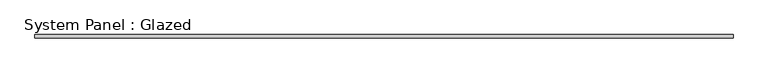
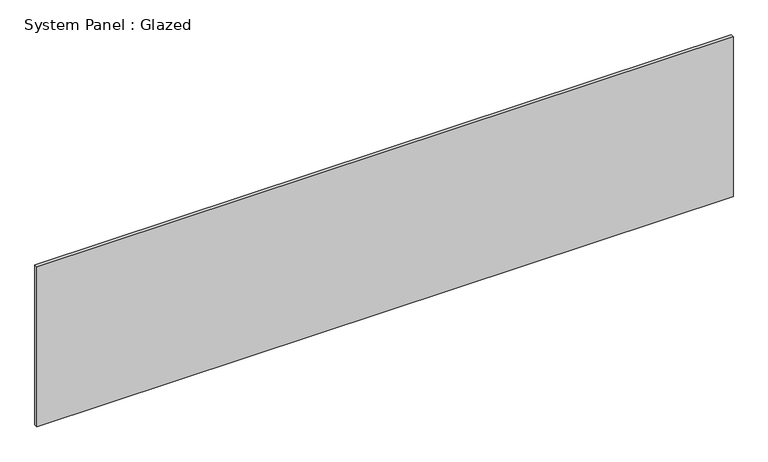
"""IFC4 building model written with IfcOpenShell, lengths in millimetres: plate geometry, System Panel : Glazed."""

from ifc_helpers import new_model, si_unit, origin, origin_with_axes, place, context, project, spatial, polyline, outline, extrude, source, transform, mapped, element, save


def system_panel_glazed_a1bdd1fe(model_context):
    return source(origin(), model_context, "Body", "SweptSolid", [
        extrude(outline(polyline([(2510.4034, 19.05), (-2510.4034, 19.05), (-2510.4034, 44.45), (2510.4034, 44.45), (2510.4034, 19.05)])), origin_with_axes(), (0.0, 0.0, 1.0), 1219.2),
    ])


if __name__ == "__main__":
    model = new_model("IFC4")
    model_context = context("Model", 3, world=origin())
    ifc_project = project(units=[si_unit("LENGTHUNIT", "METRE", prefix="MILLI")], contexts=[model_context])
    site = spatial("IfcSite", under=ifc_project)
    building = spatial("IfcBuilding", under=site)
    placement = place(None, origin())
    system_panel_glazed_shape = system_panel_glazed_a1bdd1fe(model_context)
    element("IfcPlate", 1, ObjectType="System Panel : Glazed", at=placement, inside=building, context=model_context, shape_type="MappedRepresentation", body=[
        mapped(system_panel_glazed_shape, transform((0.0, 0.0, 0.0), x_axis=(1.0, 0.0, 0.0), y_axis=(0.0, 1.0, 0.0), z_axis=(0.0, 0.0, 1.0))),
    ])
    save(model, "model.ifc")

# Revit data of these elements
# Type "System Panel : Glazed"
#   Construction Type Id = "GSP4R"
#   Analytic Construction = "1/8 in Pilkington single glazing"
#   Visual Light Transmittance = 0.9
#   Solar Heat Gain Coefficient = 0.86
#   Heat Transfer Coefficient (U) = 1.18115 BTU/(h·ft²·°F)
# Element 1 (IfcPlate, "System Panel : Glazed")
#   Materials on its faces: "Glass"
# Materials
#   "Glass": class "Glass", colour RGB 0 128 192, transparency 0.75, Description = "Soda Lime Glass", Cost = 0
